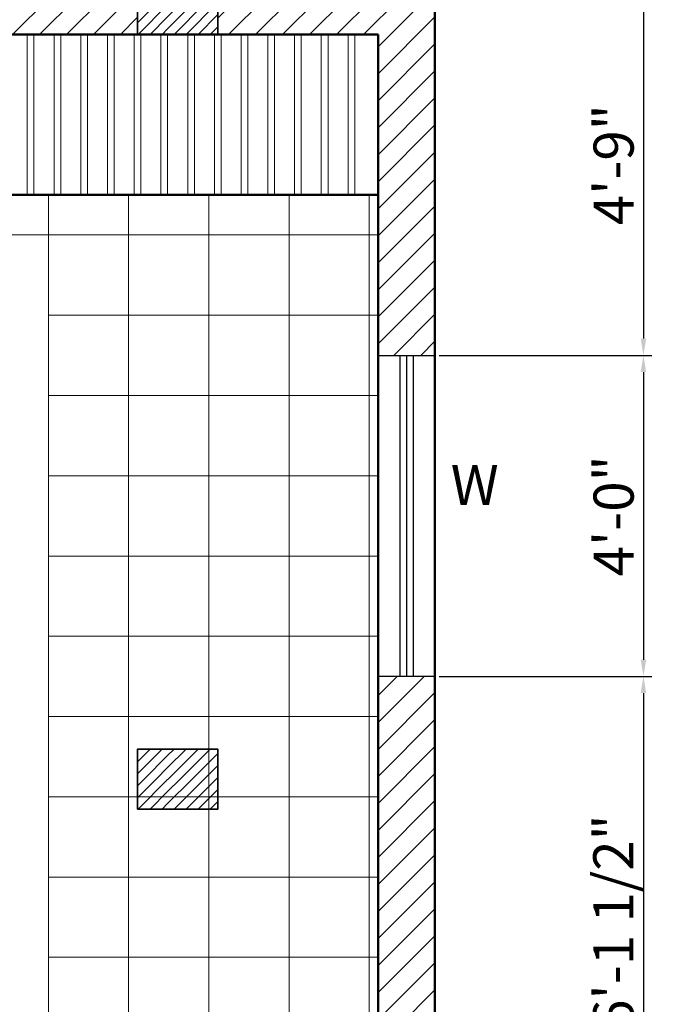
# Model space of a CAD drawing. Units: millimetres. Extents: x 225995 to 227247, y 225507 to 226008.
# Tile 9 of 23: x 226504 to 226602, y 225780 to 225927. Entities that reach past the tile are written whole.
import ezdxf

# ---------------------------------------------------------------- set-up
doc = ezdxf.new("R2010")
doc.units = ezdxf.units.MM
for name, color, linetype, lineweight in [('A-ANNO-DIMS', 2, 'Continuous', 18), ('A-ANNO-TEXT', 3, 'Continuous', 18), ('A-COLS', 40, 'Continuous', 35), ('A-FLOR-PATT', 8, 'Continuous', 13), ('A-FURN', 9, 'Continuous', 18), ('A-GLAZ', 4, 'Continuous', 25), ('A-WALL', 7, 'Continuous', 50), ('A-WALL-PATT', 8, 'Continuous', 13)]:
    doc.layers.add(name, color=color, linetype=linetype, lineweight=lineweight)
doc.styles.get("Standard").update_dxf_attribs({"font": 'arial.ttf'})
doc.dimstyles.new('ISO-25', dxfattribs={"dimtxt": 6, "dimasz": 2.5, "dimexe": 1.25, "dimexo": 0.625, "dimtad": 1, "dimdec": 0, "dimlunit": 3, "dimtxsty": 'Standard', "dimcen": 2.5, "dimadec": 0, "dimazin": 0, "dimtfac": 1, "dimtdec": 0, "dimtmove": 0, "dimatfit": 3, "dimfxl": 1, "dimarcsym": 0})
pattern_1 = [(45, (141, 118.1362), (-0.898025612, 0.898025612), [])]
pattern_2 = [(45, (141, 234), (-0.898025612, 0.898025612), [])]

# ---------------------------------------------------------------- blocks, each defined once
blk = doc.blocks.new('*D99')
at = {"layer": 'A-ANNO-DIMS', "color": 0, "lineweight": -2, "transparency": 16777216}
for p, q in [((226566.5, 225933.77), (226598.33, 225933.77)), ((226597.08, 225931.27), (226597.08, 225879.27)), ((226566.5, 225876.77), (226598.33, 225876.77))]:
    blk.add_line(p, q, dxfattribs=at)
at = {"layer": 'A-ANNO-DIMS', "color": 0, "transparency": 16777216}
for points in [[(226596.66, 225931.27), (226597.49, 225931.27), (226597.08, 225933.77)], [(226596.66, 225879.27), (226597.49, 225879.27), (226597.08, 225876.77)]]:
    blk.add_solid(points, dxfattribs=at)
at = {"layer": 'Defpoints', "color": 0, "transparency": 16777216}
for p in [(226565.88, 225933.77), (226565.88, 225876.77), (226597.08, 225876.77)]:
    blk.add_point(p, dxfattribs=at)
at = {"layer": 'A-ANNO-DIMS', "color": 0, "transparency": 16777216, "insert": (226593.39, 225905.27), "char_height": 6, "attachment_point": 5, "rotation": 90}
blk.add_mtext('4\'-9"', dxfattribs=at)
blk = doc.blocks.new('*D100')
at = {"layer": 'A-ANNO-DIMS', "color": 0, "lineweight": -2, "transparency": 16777216}
for p, q in [((226566.5, 225876.77), (226598.33, 225876.77)), ((226597.08, 225874.27), (226597.08, 225831.27)), ((226566.5, 225828.77), (226598.33, 225828.77))]:
    blk.add_line(p, q, dxfattribs=at)
at = {"layer": 'A-ANNO-DIMS', "color": 0, "transparency": 16777216}
for points in [[(226596.66, 225874.27), (226597.49, 225874.27), (226597.08, 225876.77)], [(226596.66, 225831.27), (226597.49, 225831.27), (226597.08, 225828.77)]]:
    blk.add_solid(points, dxfattribs=at)
at = {"layer": 'Defpoints', "color": 0, "transparency": 16777216}
for p in [(226565.88, 225876.77), (226565.88, 225828.77), (226597.08, 225828.77)]:
    blk.add_point(p, dxfattribs=at)
at = {"layer": 'A-ANNO-DIMS', "color": 0, "transparency": 16777216, "insert": (226593.39, 225852.77), "char_height": 6, "attachment_point": 5, "rotation": 90}
blk.add_mtext('4\'-0"', dxfattribs=at)
blk = doc.blocks.new('*D101')
at = {"layer": 'A-ANNO-DIMS', "color": 0, "lineweight": -2, "transparency": 16777216}
for p, q in [((226566.5, 225828.77), (226598.33, 225828.77)), ((226597.08, 225826.27), (226597.08, 225757.77)), ((226566.5, 225755.27), (226598.33, 225755.27))]:
    blk.add_line(p, q, dxfattribs=at)
at = {"layer": 'A-ANNO-DIMS', "color": 0, "transparency": 16777216}
for points in [[(226596.66, 225826.27), (226597.49, 225826.27), (226597.08, 225828.77)], [(226596.66, 225757.77), (226597.49, 225757.77), (226597.08, 225755.27)]]:
    blk.add_solid(points, dxfattribs=at)
at = {"layer": 'Defpoints', "color": 0, "transparency": 16777216}
for p in [(226565.88, 225828.77), (226565.88, 225755.27), (226597.08, 225755.27)]:
    blk.add_point(p, dxfattribs=at)
at = {"layer": 'A-ANNO-DIMS', "color": 0, "transparency": 16777216, "insert": (226593.35, 225792.02), "char_height": 6, "attachment_point": 5, "rotation": 90}
blk.add_mtext('6\'-1 1/2"', dxfattribs=at)

msp = doc.modelspace()

# ---------------------------------------------------------------- hatches: boundary and pattern name
at = {"layer": 'A-WALL-PATT'}
h = msp.add_hatch(dxfattribs=at)
h.set_pattern_fill('ANSI31', color=256, scale=0.9)
h.paths.add_polyline_path([(226521.38, 225933.77), (226392.38, 225933.77), (226392.38, 225924.77), (226521.38, 225924.77)])
h = msp.add_hatch(dxfattribs=at)
h.set_pattern_fill('ANSI31', color=256, scale=0.9)
h.paths.add_polyline_path([(226565.88, 225933.77), (226533.38, 225933.77), (226533.38, 225924.77), (226557.38, 225924.77), (226557.38, 225876.77), (226565.88, 225876.77)])
h = msp.add_hatch(dxfattribs=at)
h.set_pattern_fill('ANSI31', color=256, scale=0.4)
h.set_pattern_definition(pattern_2)
h.paths.add_polyline_path([(226525.88, 225929.27), (226521.38, 225929.27), (226521.38, 225924.77), (226525.88, 225924.77)])
h = msp.add_hatch(dxfattribs=at)
h.set_pattern_fill('ANSI31', color=256, scale=0.4)
h.set_pattern_definition(pattern_2)
h.paths.add_polyline_path([(226533.38, 225929.27), (226525.88, 225929.27), (226525.88, 225924.77), (226533.38, 225924.77)])
h = msp.add_hatch(dxfattribs=at)
h.set_pattern_fill('ANSI31', color=256, scale=0.9)
h.paths.add_polyline_path([(226565.88, 225828.77), (226557.38, 225828.77), (226557.38, 225755.27), (226565.88, 225755.27)])
h = msp.add_hatch(dxfattribs=at)
h.set_pattern_fill('ANSI31', color=256, scale=0.4)
h.set_pattern_definition(pattern_1)
h.paths.add_polyline_path([(226525.88, 225817.91), (226521.38, 225817.91), (226521.38, 225813.41), (226525.88, 225813.41)])
h = msp.add_hatch(dxfattribs=at)
h.set_pattern_fill('ANSI31', color=256, scale=0.4)
h.set_pattern_definition(pattern_1)
h.paths.add_polyline_path([(226533.38, 225817.91), (226525.88, 225817.91), (226525.88, 225813.41), (226533.38, 225813.41)])
h = msp.add_hatch(dxfattribs=at)
h.set_pattern_fill('ANSI31', color=256, scale=0.4)
h.set_pattern_definition(pattern_1)
h.paths.add_polyline_path([(226525.88, 225813.41), (226521.38, 225813.41), (226521.38, 225808.91), (226525.88, 225808.91)])
h = msp.add_hatch(dxfattribs=at)
h.set_pattern_fill('ANSI31', color=256, scale=0.4)
h.set_pattern_definition(pattern_1)
h.paths.add_polyline_path([(226533.38, 225813.41), (226525.88, 225813.41), (226525.88, 225808.91), (226533.38, 225808.91)])

# ---------------------------------------------------------------- linework, layer by layer
at = {"layer": 'A-COLS'}
for points in [[(226521.38, 225924.77), (226521.38, 225933.77), (226533.38, 225933.77), (226533.38, 225924.77)], [(226521.38, 225808.91), (226521.38, 225817.91), (226533.38, 225817.91), (226533.38, 225808.91)]]:
    msp.add_lwpolyline(points, close=True, dxfattribs=at)
at = {"layer": 'A-FLOR-PATT'}
for p, q in [((226508.05, 225900.77), (226508.05, 225695.27)), ((226520.05, 225900.77), (226520.05, 225695.27)), ((226532.05, 225900.77), (226532.05, 225699.77)), ((226544.05, 225900.77), (226544.05, 225695.27)), ((226384.88, 225894.77), (226557.38, 225894.77)), ((226508.05, 225882.77), (226557.38, 225882.77)), ((226508.05, 225870.77), (226557.38, 225870.77)), ((226508.05, 225858.77), (226557.38, 225858.77)), ((226508.05, 225846.77), (226557.38, 225846.77)), ((226508.05, 225834.77), (226557.38, 225834.77)), ((226508.05, 225822.77), (226557.38, 225822.77)), ((226508.05, 225810.77), (226557.38, 225810.77)), ((226508.05, 225798.77), (226557.38, 225798.77)), ((226508.05, 225786.77), (226557.38, 225786.77))]:
    msp.add_line(p, q, dxfattribs=at)
at = {"layer": 'A-FURN'}
for p, q in [((226504.88, 225900.77), (226504.88, 225924.77)), ((226505.88, 225900.77), (226505.88, 225924.77)), ((226508.88, 225900.77), (226508.88, 225924.77)), ((226509.88, 225900.77), (226509.88, 225924.77)), ((226512.88, 225900.77), (226512.88, 225924.77)), ((226513.88, 225900.77), (226513.88, 225924.77)), ((226516.88, 225900.77), (226516.88, 225924.77)), ((226517.88, 225900.77), (226517.88, 225924.77)), ((226520.88, 225900.77), (226520.88, 225924.77)), ((226521.88, 225900.77), (226521.88, 225924.77)), ((226524.88, 225900.77), (226524.88, 225924.77)), ((226525.88, 225900.77), (226525.88, 225924.77)), ((226528.88, 225900.77), (226528.88, 225924.77)), ((226529.88, 225900.77), (226529.88, 225924.77)), ((226532.88, 225900.77), (226532.88, 225924.77)), ((226533.88, 225900.77), (226533.88, 225924.77)), ((226536.88, 225900.77), (226536.88, 225924.77)), ((226537.88, 225900.77), (226537.88, 225924.77)), ((226540.88, 225900.77), (226540.88, 225924.77)), ((226541.88, 225900.77), (226541.88, 225924.77)), ((226544.88, 225900.77), (226544.88, 225924.77)), ((226545.88, 225900.77), (226545.88, 225924.77)), ((226548.88, 225900.77), (226548.88, 225924.77)), ((226549.88, 225900.77), (226549.88, 225924.77)), ((226552.88, 225900.77), (226552.88, 225924.77)), ((226553.88, 225900.77), (226553.88, 225924.77)), ((226556.05, 225900.77), (226556.05, 225695.27)), ((226557.38, 225876.77), (226565.88, 225876.77)), ((226557.38, 225828.77), (226565.88, 225828.77))]:
    msp.add_line(p, q, dxfattribs=at)
at = {"layer": 'A-GLAZ'}
for p, q in [((226560.63, 225876.77), (226560.63, 225828.77)), ((226561.63, 225876.77), (226561.63, 225828.77)), ((226562.63, 225876.77), (226562.63, 225828.77))]:
    msp.add_line(p, q, dxfattribs=at)
msp.add_lwpolyline([(226557.38, 225876.77), (226565.88, 225876.77), (226565.88, 225828.77), (226557.38, 225828.77)], close=True, dxfattribs=at)
at = {"layer": 'A-WALL'}
for p, q in [((226565.88, 225933.77), (226565.88, 225570.77)), ((226565.88, 225570.77), (226565.88, 225933.77)), ((226236.38, 225924.77), (226557.38, 225924.77)), ((226384.88, 225924.77), (226557.38, 225924.77)), ((226557.38, 225695.27), (226557.38, 225924.77)), ((226557.38, 225924.77), (226557.38, 225579.77)), ((226384.88, 225900.77), (226557.38, 225900.77))]:
    msp.add_line(p, q, dxfattribs=at)

# ---------------------------------------------------------------- texts
at = {"layer": 'A-ANNO-TEXT', "insert": (226562.74, 225860.39), "char_height": 6, "attachment_point": 1}
msp.add_mtext_dynamic_manual_height_columns('   W', width=24.8115, gutter_width=12.5, heights=[0], dxfattribs=at)

# ---------------------------------------------------------------- dimensions: what is measured, and where the dimension line sits
at = {"layer": 'A-ANNO-DIMS'}
for base, p1, p2, picture, middle in [((226597.08, 225876.77), (226565.88, 225933.77), (226565.88, 225876.77), '*D99', (226593.39, 225905.27)), ((226597.08, 225828.77), (226565.88, 225876.77), (226565.88, 225828.77), '*D100', (226593.39, 225852.77)), ((226597.08, 225755.27), (226565.88, 225828.77), (226565.88, 225755.27), '*D101', (226593.35, 225792.02))]:
    dim = msp.add_linear_dim(base=base, p1=p1, p2=p2, angle=90, dimstyle='ISO-25', override={"dimdec": 1, "dimlfac": 1, "dimrnd": 0, "dimzin": 1, "dimdsep": 46, "dimlunit": 4, "dimfrac": 2}, dxfattribs=at)
    dim.commit()
    dim.dimension.update_dxf_attribs({"geometry": picture, "text_midpoint": middle})

doc.saveas('drawing.dxf')
